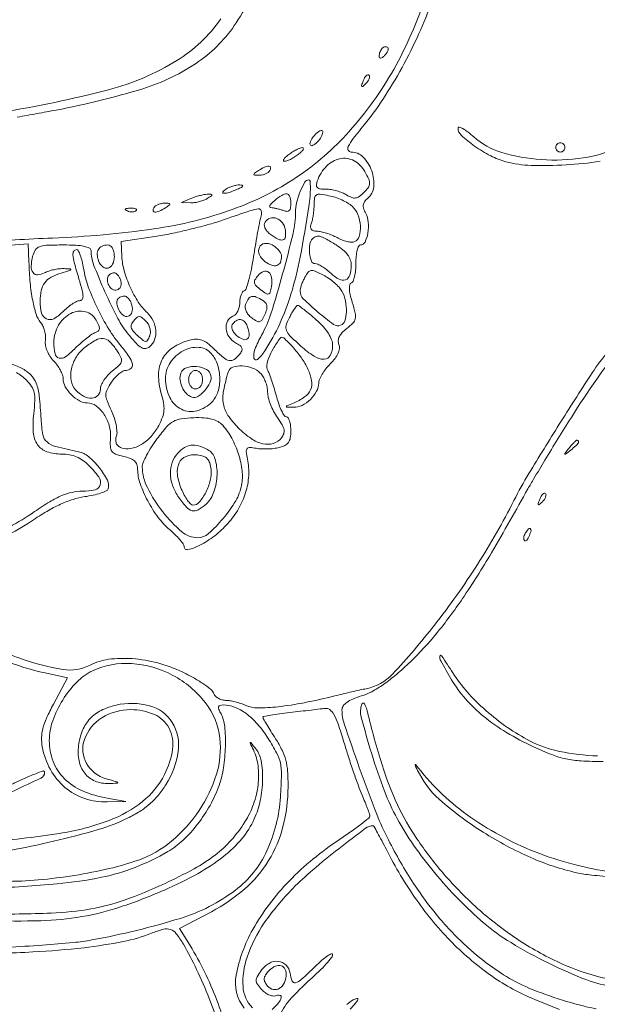
# Model space of a CAD drawing. Units: inches. Extents: x 2656 to 9931, y 1941 to 3068.
# Tile 34 of 46: x 2845.52 to 2854.27, y 2952.23 to 2967.13. Entities that reach past the tile are written whole.
import ezdxf

# ---------------------------------------------------------------- set-up
doc = ezdxf.new("R2010")
doc.units = ezdxf.units.IN
doc.layers.add('A-ANNO-DIMS', color=2, linetype='Continuous', lineweight=18)
doc.layers.add('A-ELEV-ORN', color=8, linetype='Continuous', lineweight=13)
doc.styles.get("Standard").update_dxf_attribs({"font": 'arial.ttf'})
doc.dimstyles.new('ISO-25', dxfattribs={"dimtxt": 6, "dimasz": 2.5, "dimexe": 1.25, "dimexo": 0.625, "dimtad": 1, "dimdec": 0, "dimlunit": 3, "dimtxsty": 'Standard', "dimcen": 2.5, "dimadec": 0, "dimazin": 0, "dimtfac": 1, "dimtdec": 0, "dimtmove": 0, "dimatfit": 3, "dimfxl": 1, "dimarcsym": 0})

# ---------------------------------------------------------------- blocks, each defined once
blk = doc.blocks.new('*D151')
at = {"layer": 'A-ANNO-DIMS', "color": 0, "lineweight": -2, "transparency": 16777216}
for p, q in [((2829.546, 2956.424), (2829.546, 2703.709)), ((2867.059, 2955.98), (2867.059, 2703.709)), ((2832.046, 2704.959), (2864.559, 2704.959))]:
    blk.add_line(p, q, dxfattribs=at)
at = {"layer": 'A-ANNO-DIMS', "color": 0, "transparency": 16777216}
for points in [[(2832.046, 2705.376), (2832.046, 2704.543), (2829.546, 2704.959)], [(2864.559, 2705.376), (2864.559, 2704.543), (2867.059, 2704.959)]]:
    blk.add_solid(points, dxfattribs=at)
at = {"layer": 'Defpoints', "color": 0, "transparency": 16777216}
for p in [(2829.546, 2957.049), (2867.059, 2956.605), (2867.059, 2704.959)]:
    blk.add_point(p, dxfattribs=at)
at = {"layer": 'A-ANNO-DIMS', "color": 0, "transparency": 16777216, "insert": (2848.302, 2708.689), "char_height": 6, "attachment_point": 5}
blk.add_mtext('3\'-1 1/2"', dxfattribs=at)
blk = doc.blocks.new('*D152')
at = {"layer": 'A-ANNO-DIMS', "color": 0, "lineweight": -2, "transparency": 16777216}
for p, q in [((2847.28, 2990.828), (2707.323, 2990.828)), ((2708.573, 2988.328), (2708.573, 2952.971)), ((2847.248, 2950.471), (2707.323, 2950.471))]:
    blk.add_line(p, q, dxfattribs=at)
at = {"layer": 'A-ANNO-DIMS', "color": 0, "transparency": 16777216}
for points in [[(2708.156, 2988.328), (2708.989, 2988.328), (2708.573, 2990.828)], [(2708.156, 2952.971), (2708.989, 2952.971), (2708.573, 2950.471)]]:
    blk.add_solid(points, dxfattribs=at)
at = {"layer": 'Defpoints', "color": 0, "transparency": 16777216}
for p in [(2847.905, 2990.828), (2708.573, 2950.471), (2847.873, 2950.471)]:
    blk.add_point(p, dxfattribs=at)
at = {"layer": 'A-ANNO-DIMS', "color": 0, "transparency": 16777216, "insert": (2704.843, 2970.649), "char_height": 6, "attachment_point": 5, "rotation": 90}
blk.add_mtext('3\'-4 1/2"', dxfattribs=at)
blk = doc.blocks.new('*D153')
at = {"layer": 'A-ANNO-DIMS', "color": 0, "lineweight": -2, "transparency": 16777216}
for p, q in [((2826.64, 2993.722), (2826.64, 2703.709)), ((2829.546, 2956.424), (2829.546, 2703.709)), ((2824.14, 2704.959), (2821.64, 2704.959)), ((2826.64, 2704.959), (2829.546, 2704.959)), ((2832.046, 2704.959), (2851.745, 2704.959))]:
    blk.add_line(p, q, dxfattribs=at)
at = {"layer": 'A-ANNO-DIMS', "color": 0, "transparency": 16777216}
for points in [[(2824.14, 2705.376), (2824.14, 2704.543), (2826.64, 2704.959)], [(2832.046, 2705.376), (2832.046, 2704.543), (2829.546, 2704.959)]]:
    blk.add_solid(points, dxfattribs=at)
at = {"layer": 'Defpoints', "color": 0, "transparency": 16777216}
for p in [(2826.64, 2994.347), (2829.546, 2957.049), (2829.546, 2704.959)]:
    blk.add_point(p, dxfattribs=at)
at = {"layer": 'A-ANNO-DIMS', "color": 0, "transparency": 16777216, "insert": (2843.145, 2708.65), "char_height": 6, "attachment_point": 5}
blk.add_mtext('0\'-3"', dxfattribs=at)
blk = doc.blocks.new('*D154')
at = {"layer": 'A-ANNO-DIMS', "color": 0, "lineweight": -2, "transparency": 16777216}
for p, q in [((2708.573, 2996.847), (2708.573, 2999.347)), ((2826.015, 2994.347), (2707.323, 2994.347)), ((2708.573, 2994.347), (2708.573, 2990.828)), ((2847.28, 2990.828), (2707.323, 2990.828)), ((2708.573, 2988.328), (2708.573, 2954.647))]:
    blk.add_line(p, q, dxfattribs=at)
at = {"layer": 'A-ANNO-DIMS', "color": 0, "transparency": 16777216}
for points in [[(2708.156, 2996.847), (2708.989, 2996.847), (2708.573, 2994.347)], [(2708.156, 2988.328), (2708.989, 2988.328), (2708.573, 2990.828)]]:
    blk.add_solid(points, dxfattribs=at)
at = {"layer": 'Defpoints', "color": 0, "transparency": 16777216}
for p in [(2826.64, 2994.347), (2708.573, 2990.828), (2847.905, 2990.828)]:
    blk.add_point(p, dxfattribs=at)
at = {"layer": 'A-ANNO-DIMS', "color": 0, "transparency": 16777216, "insert": (2704.843, 2970.237), "char_height": 6, "attachment_point": 5, "rotation": 90}
blk.add_mtext('0\'-3 1/2"', dxfattribs=at)

msp = doc.modelspace()

# ---------------------------------------------------------------- linework, layer by layer
at = {"layer": 'A-ELEV-ORN'}
for points in [[(2845.488, 2965.66, 0.001937), (2845.785, 2965.713, 0.002024), (2846.077, 2965.767, 0.02762), (2847.387, 2966.09, 0.077708), (2848.233, 2966.501, 0.09773), (2848.802, 2967.089, 0.062193), (2849.216, 2967.949, 0.059261)], [(2851.685, 2967.523, -0.020457), (2851.452, 2966.917, -0.026412), (2851.187, 2966.383, -0.02755), (2850.877, 2965.898, -0.026024), (2850.511, 2965.441, -0.064031), (2849.714, 2964.749, -0.060807), (2848.755, 2964.267, -0.050453), (2847.555, 2963.968, -0.026486), (2846.021, 2963.83, 0.014791), (2844.896, 2963.755, 0.039833)], [(2845.128, 2963.701), (2845.655, 2963.743), (2845.664, 2963.47, 0.015098), (2845.683, 2963.15, 0.025215), (2845.721, 2962.883, 0.029482), (2845.774, 2962.676, 0.096217), (2845.841, 2962.552, -0.067329), (2845.876, 2962.497, -0.041313), (2845.901, 2962.425, -0.040734), (2845.915, 2962.348, -0.056588), (2845.914, 2962.278, 0.07899), (2845.916, 2962.204, 0.049795), (2845.94, 2962.121, 0.047545), (2845.982, 2962.04, 0.052886), (2846.038, 2961.971, -0.039614), (2846.093, 2961.906, -0.035337), (2846.14, 2961.83, -0.037086), (2846.173, 2961.756, -0.084565), (2846.183, 2961.696, 0.131359), (2846.214, 2961.579, 0.066289), (2846.307, 2961.458, 0.066248), (2846.43, 2961.365, 0.130477), (2846.547, 2961.334, -0.158296), (2846.68, 2961.29, -0.088368), (2846.799, 2961.166, -0.079038), (2846.879, 2960.993, -0.085713), (2846.899, 2960.808, 0.027358), (2846.897, 2960.673, 0.142212), (2846.92, 2960.603, 0.154173), (2846.977, 2960.56, 0.033889), (2847.095, 2960.525, -0.037614), (2847.196, 2960.495, -0.09597), (2847.261, 2960.455, -0.121453), (2847.297, 2960.4, -0.082169), (2847.31, 2960.326, 0.083183), (2847.347, 2960.114, 0.036336), (2847.463, 2959.852, 0.036114), (2847.62, 2959.601, 0.059955), (2847.791, 2959.419, -0.017475), (2847.875, 2959.342, -0.02288), (2847.947, 2959.266, -0.021356), (2847.999, 2959.2, -0.157402), (2848.012, 2959.161, 0.482329), (2848.072, 2959.113, 0.063629), (2848.251, 2959.179, 0.044846), (2848.476, 2959.323, 0.043978), (2848.673, 2959.507, 0.051485), (2848.837, 2959.731, 0.057599), (2848.945, 2959.976, 0.059909), (2848.991, 2960.23, 0.064303), (2848.973, 2960.482, -0.019043), (2848.955, 2960.597, -0.200466), (2848.967, 2960.643, -0.248203), (2849.007, 2960.66, -0.029106), (2849.104, 2960.647, 0.03518), (2849.182, 2960.638, 0.020558), (2849.277, 2960.637, 0.020491), (2849.372, 2960.644, 0.032499), (2849.452, 2960.659, 0.054058), (2849.54, 2960.691, 0.125687), (2849.593, 2960.737, 0.113297), (2849.621, 2960.806, 0.039391), (2849.629, 2960.913, 0.030528), (2849.624, 2960.993, 0.047396), (2849.609, 2961.061, 0.060348), (2849.588, 2961.108, 0.260189), (2849.562, 2961.123, -0.25441), (2849.531, 2961.139, -0.029188), (2849.491, 2961.21, -0.029502), (2849.45, 2961.307, -0.019772), (2849.415, 2961.422, 0.007204), (2849.38, 2961.544, 0.007421), (2849.342, 2961.664, 0.007216), (2849.307, 2961.767, 0.03111), (2849.281, 2961.826, -0.151629), (2849.267, 2961.906, -0.058986), (2849.295, 2962.016, -0.043726), (2849.361, 2962.151, -0.02136), (2849.467, 2962.312, -0.446077), (2849.521, 2962.318, -0.02582), (2849.653, 2962.186, -0.030731), (2849.789, 2962.016, -0.042151), (2849.887, 2961.847, -0.065624), (2849.943, 2961.672, -0.146964), (2849.928, 2961.534, -0.139685), (2849.838, 2961.424, -0.057016), (2849.667, 2961.33, 0.002265), (2849.567, 2961.289, 0.321547), (2849.561, 2961.279, 0.38279), (2849.569, 2961.271, 0.002608), (2849.671, 2961.268, 0.125541), (2849.798, 2961.296, 0.074808), (2849.925, 2961.386, 0.074894), (2850.019, 2961.51, 0.12662), (2850.051, 2961.635, -0.104017), (2850.063, 2961.691, -0.032384), (2850.103, 2961.767, -0.030802), (2850.159, 2961.849, -0.029548), (2850.226, 2961.924, 0.033876), (2850.298, 2962.007, 0.058545), (2850.344, 2962.085, 0.074645), (2850.364, 2962.156, 0.121698), (2850.356, 2962.218, -0.110816), (2850.347, 2962.277, -0.096177), (2850.364, 2962.338, -0.075761), (2850.407, 2962.399, -0.040897), (2850.476, 2962.461, 0.036829), (2850.568, 2962.542, 0.143956), (2850.604, 2962.608, 0.109376), (2850.603, 2962.693, 0.016954), (2850.559, 2962.857, -0.018723), (2850.527, 2962.973, -0.04405), (2850.515, 2963.062, -0.066055), (2850.52, 2963.124, -0.262755), (2850.545, 2963.151, 0.222508), (2850.572, 2963.176, 0.035254), (2850.594, 2963.248, 0.033397), (2850.609, 2963.342, 0.023544), (2850.614, 2963.449, -0.023642), (2850.619, 2963.555, -0.037732), (2850.634, 2963.644, -0.043931), (2850.656, 2963.708, -0.295632), (2850.683, 2963.725, 0.29178), (2850.752, 2963.769, 0.067923), (2850.794, 2963.906, 0.061292), (2850.801, 2964.071, 0.102977), (2850.762, 2964.203, -0.042589), (2850.731, 2964.276, -0.112846), (2850.725, 2964.332, -0.126957), (2850.745, 2964.38, -0.061228), (2850.791, 2964.43, 0.199048), (2850.883, 2964.604, 0.109415), (2850.853, 2964.848, 0.109618), (2850.722, 2965.056, 0.200184), (2850.54, 2965.132, -0.298413), (2850.498, 2965.159, -0.222638), (2850.499, 2965.217, -0.048145), (2850.573, 2965.335, -0.006113), (2850.761, 2965.571, 0.02817), (2851.056, 2965.98, 0.01926), (2851.346, 2966.474, 0.019246), (2851.598, 2966.989, 0.02788), (2851.777, 2967.464, -0.014526)], [(2848.567, 2967.146, -0.103766), (2847.903, 2966.516, -0.074462), (2846.868, 2966.075, -0.024075), (2845.233, 2965.732, 0.023987)], [(2854.6, 2965.209, -0.074881), (2854.055, 2965.042, -0.054125), (2853.419, 2965.017, -0.0559), (2852.822, 2965.125, -0.107645), (2852.399, 2965.36, 0.015979), (2852.308, 2965.435, 0.033182), (2852.231, 2965.486, 0.053925), (2852.178, 2965.509, 0.507729), (2852.161, 2965.497, 0.210529), (2852.211, 2965.383, 0.031431), (2852.411, 2965.222, 0.034984), (2852.655, 2965.075, 0.052971), (2852.885, 2964.985, 0.058384), (2853.265, 2964.929, 0.022857), (2853.796, 2964.937, 0.021823), (2854.311, 2964.991, 0.083985)], [(2854.249, 2952.161, -0.023008), (2853.739, 2952.294, -0.023068), (2853.234, 2952.477, -0.042969), (2852.847, 2952.678, -0.040395), (2852.342, 2953.059, -0.035477), (2851.881, 2953.532, -0.033085), (2851.462, 2954.099, -0.026219), (2851.085, 2954.761, -0.024093), (2850.904, 2955.171, -0.007059), (2850.665, 2955.816, -0.00416), (2850.438, 2956.475, -0.081132), (2850.403, 2956.687, -0.152749), (2850.422, 2956.747, -0.08592), (2850.475, 2956.801, -0.058118), (2850.566, 2956.852, -0.024591), (2850.697, 2956.898, 0.052149), (2850.853, 2956.963, 0.027424), (2851.031, 2957.073, 0.023518), (2851.227, 2957.224, 0.015475), (2851.438, 2957.415, 0.030449), (2851.835, 2957.846, 0.021735), (2852.228, 2958.372, 0.016396), (2852.666, 2959.066, 0.006747), (2853.217, 2960.032, -0.008584), (2853.308, 2960.189, -0.001712), (2853.475, 2960.467, -0.001811), (2853.671, 2960.788, -0.001687), (2853.875, 2961.115, -0.028373), (2854.681, 2962.254, -0.056082)], [(2854.396, 2962.072, 0.025999), (2854.163, 2961.749, 0.003163), (2853.692, 2961.01, 0.003538), (2853.233, 2960.266, 0.019761), (2853.006, 2959.857, -0.025293), (2852.455, 2958.89, -0.024226), (2851.802, 2957.969, -0.021134), (2851.169, 2957.229, -0.158603), (2850.771, 2957.008, 0.005641), (2850.677, 2956.989, 0.002373), (2850.553, 2956.961, 0.002347), (2850.419, 2956.93, 0.003055), (2850.297, 2956.9, -0.012629), (2849.829, 2956.795, -0.021947), (2849.435, 2956.735, -0.024664), (2849.125, 2956.717, -0.10946), (2848.948, 2956.755, 0.02618), (2848.873, 2956.784, 0.019467), (2848.787, 2956.809, 0.019793), (2848.705, 2956.827, 0.041477), (2848.639, 2956.832, -0.074507), (2848.582, 2956.841, -0.064432), (2848.528, 2956.866, -0.066856), (2848.483, 2956.902, -0.09592), (2848.456, 2956.946, 0.135164), (2848.415, 2957.001, 0.019232), (2848.299, 2957.085, 0.020724), (2848.151, 2957.176, 0.016328), (2847.983, 2957.262, 0.045412), (2847.613, 2957.398, 0.046726), (2847.227, 2957.463, 0.050582), (2846.871, 2957.453, 0.0883), (2846.59, 2957.365, -0.163294), (2846.18, 2957.3, -0.042657), (2845.525, 2957.468, -0.038553), (2844.769, 2957.801, -0.030663)], [(2845.302, 2959.316, 0.03899), (2845.705, 2959.546, -0.016354), (2845.935, 2959.692, -0.025518), (2846.142, 2959.8, -0.029603), (2846.332, 2959.874, -0.042475), (2846.508, 2959.915, 0.018492), (2846.637, 2959.938, 0.026143), (2846.749, 2959.969, 0.024598), (2846.835, 2960.002, 0.211487), (2846.862, 2960.032, 0.2024), (2846.852, 2960.165, 0.048072), (2846.729, 2960.354, 0.04877), (2846.565, 2960.522, 0.126447), (2846.414, 2960.596, -0.011877), (2846.069, 2960.674, -0.117882), (2845.938, 2960.743, -0.170367), (2845.875, 2960.853, -0.031647), (2845.848, 2961.089, 0.01358), (2845.82, 2961.439, 0.064726), (2845.773, 2961.633, 0.107185), (2845.691, 2961.759, 0.075435), (2845.553, 2961.859, 0.057839), (2845.366, 2961.93, 0.180103)], [(2845.477, 2961.793, -0.065835), (2845.629, 2961.677, -0.052375), (2845.705, 2961.582, -0.092126), (2845.744, 2961.49, -0.065516), (2845.753, 2961.369, -0.016207), (2845.736, 2961.17, 0.048024), (2845.73, 2960.887, 0.134535), (2845.796, 2960.701, 0.162378), (2845.937, 2960.596, 0.079646), (2846.162, 2960.56, -0.046996), (2846.277, 2960.549, -0.052481), (2846.384, 2960.517, -0.052054), (2846.482, 2960.463, -0.044979), (2846.573, 2960.387, -0.040846), (2846.721, 2960.213, -0.222133), (2846.743, 2960.095, -0.278389), (2846.666, 2960.02, -0.058192), (2846.472, 2959.997, 0.053728), (2846.317, 2959.98, 0.047138), (2846.161, 2959.931, 0.035355), (2845.981, 2959.839, 0.01398), (2845.748, 2959.688, -0.025269), (2845.366, 2959.454, -0.03501)], [(2845.269, 2957.445, 0.045204), (2845.91, 2957.246), (2846.249, 2957.173), (2846.036, 2956.774, 0.015297), (2845.93, 2956.562, 0.043542), (2845.875, 2956.406, 0.058138), (2845.856, 2956.271, 0.050737), (2845.867, 2956.129, 0.08076), (2845.989, 2955.785, 0.091523), (2846.21, 2955.515, 0.093905), (2846.508, 2955.346, 0.090131), (2846.851, 2955.294), (2847.132, 2955.302), (2846.851, 2955.35, -0.060063), (2846.476, 2955.461, -0.094302), (2846.199, 2955.649, -0.105744), (2846.031, 2955.908, -0.092677), (2845.973, 2956.226, -0.084233), (2846.025, 2956.521, -0.053759), (2846.176, 2956.836, -0.054037), (2846.389, 2957.108, -0.089289), (2846.626, 2957.278, -0.12956), (2847.218, 2957.389, -0.104076), (2847.843, 2957.21, -0.105901), (2848.334, 2956.797, -0.138836), (2848.554, 2956.257, -0.101934), (2848.503, 2955.715, -0.073419), (2848.241, 2955.163, -0.071874), (2847.824, 2954.7, -0.089033), (2847.321, 2954.414, -0.027379), (2846.877, 2954.285, -0.017773), (2846.353, 2954.182, -0.017434), (2845.806, 2954.114, -0.021563), (2845.294, 2954.091, 0.019337)], [(2854.272, 2955.99, -0.038832), (2853.696, 2956.059, -0.070977), (2853.251, 2956.215, -0.031899), (2852.908, 2956.422, -0.028892), (2852.581, 2956.678, -0.029711), (2852.297, 2956.961, -0.04108), (2852.08, 2957.248, 0.005134), (2851.912, 2957.507, 0.683993), (2851.885, 2957.501, 0.168909), (2851.898, 2957.43, 0.004262), (2852.063, 2957.142, 0.049361), (2852.273, 2956.854, 0.039427), (2852.549, 2956.589, 0.035646), (2852.893, 2956.346, 0.026402), (2853.304, 2956.127, 0.01732), (2853.578, 2956.01, 0.040071), (2853.793, 2955.946, 0.037153), (2854.024, 2955.915, 0.013073), (2854.359, 2955.904, 0.095042)], [(2845.358, 2954.556, 0.010951), (2846.035, 2954.698, 0.013876), (2846.714, 2954.876, 0.042698), (2847.157, 2955.047, 0.026486), (2847.343, 2955.151, 0.038993), (2847.494, 2955.263, 0.040467), (2847.621, 2955.394, 0.031765), (2847.737, 2955.553, 0.105705), (2847.924, 2956.058, 0.177208), (2847.832, 2956.496, 0.190205), (2847.488, 2956.75, 0.121379), (2846.985, 2956.76, 0.059498), (2846.756, 2956.679, 0.091), (2846.588, 2956.554, 0.092006), (2846.476, 2956.378, 0.062064), (2846.416, 2956.147, 0.082949), (2846.423, 2955.915, 0.11799), (2846.509, 2955.728, 0.12778), (2846.665, 2955.61, 0.107339), (2846.869, 2955.573, 0.002441), (2847.001, 2955.578, 0.534877), (2847.007, 2955.587, 0.215183), (2846.993, 2955.598, 0.001329), (2846.835, 2955.644, -0.194581), (2846.537, 2955.878, -0.218344), (2846.504, 2956.239, -0.170701), (2846.769, 2956.567, -0.139753), (2847.204, 2956.692, -0.1027), (2847.563, 2956.617, -0.172156), (2847.785, 2956.41, -0.157067), (2847.839, 2956.093, -0.082545), (2847.716, 2955.707, -0.106392), (2847.384, 2955.301, -0.078804), (2846.879, 2955.014, -0.051815), (2846.123, 2954.817, -0.017355), (2844.987, 2954.683, 0.004203)], [(2845.058, 2953.984, 0.008566), (2846.094, 2954.055, 0.029332), (2846.762, 2954.153, 0.042246), (2847.274, 2954.304, 0.039474), (2847.765, 2954.542, 0.055678), (2847.998, 2954.716, 0.039563), (2848.218, 2954.958, 0.038179), (2848.406, 2955.242, 0.04122), (2848.543, 2955.545, 0.048745), (2848.61, 2955.812, 0.030311), (2848.638, 2956.135, 0.029611), (2848.628, 2956.437, 0.100228), (2848.572, 2956.626, -0.02464), (2848.539, 2956.695, -0.156991), (2848.536, 2956.734, -0.269337), (2848.556, 2956.755, -0.072224), (2848.604, 2956.762, -0.094583), (2848.777, 2956.729, -0.065244), (2848.953, 2956.631, -0.054803), (2849.125, 2956.472, -0.035883), (2849.286, 2956.256, -0.020267), (2849.414, 2956.037, -0.07093), (2849.47, 2955.884, -0.057405), (2849.486, 2955.706, -0.010213), (2849.472, 2955.37, -0.091557), (2849.266, 2954.553, -0.123706), (2848.791, 2953.96, -0.087858), (2847.957, 2953.532, -0.029294), (2846.618, 2953.205, -0.021888), (2846.337, 2953.166, -0.00529), (2845.869, 2953.127, -0.005418), (2845.331, 2953.093, -0.005359)], [(2848.643, 2951.884, 0.023015), (2848.508, 2952.294, 0.022134), (2848.321, 2952.724, 0.024838), (2848.104, 2953.119), (2847.944, 2953.379), (2848.426, 2953.633, 0.058566), (2848.931, 2953.979, 0.075611), (2849.293, 2954.407, 0.076083), (2849.51, 2954.922, 0.060209), (2849.587, 2955.521, 0.018573), (2849.58, 2955.757, 0.046373), (2849.552, 2955.927, 0.051606), (2849.496, 2956.078, 0.028121), (2849.399, 2956.251, -0.003788), (2849.325, 2956.366, -0.005753), (2849.263, 2956.468, -0.002389), (2849.212, 2956.556, -0.131705), (2849.207, 2956.575, -0.358554), (2849.217, 2956.586, -0.003968), (2849.326, 2956.607, -0.009986), (2849.457, 2956.628, -0.006072), (2849.612, 2956.647, 0.000413), (2849.776, 2956.666, 0.000452), (2849.935, 2956.685, 0.000422), (2850.071, 2956.701, 0.002277), (2850.145, 2956.71, -0.19687), (2850.218, 2956.691, -0.102786), (2850.28, 2956.619, -0.046521), (2850.345, 2956.474, -0.008902), (2850.432, 2956.199, 0.005518), (2850.501, 2955.977, 0.004821), (2850.578, 2955.747, 0.004852), (2850.651, 2955.54, 0.014345), (2850.707, 2955.399, -0.005987), (2850.752, 2955.291, -0.008067), (2850.79, 2955.193, -0.00579), (2850.82, 2955.11, -0.082339), (2850.825, 2955.079, -0.227737), (2850.811, 2955.05, -0.005167), (2850.69, 2954.955, -0.010558), (2850.541, 2954.846, -0.006824), (2850.364, 2954.725, 0.052929), (2849.604, 2954.097, 0.065264), (2849.053, 2953.362, 0.082259), (2848.801, 2952.672, 0.216659), (2848.924, 2952.173, 0.024142)], [(2854.437, 2952.614, -0.051733), (2853.786, 2952.82, -0.039695), (2853.128, 2953.172, -0.037706), (2852.498, 2953.645, -0.035619), (2851.934, 2954.216, -0.028457), (2851.536, 2954.738, -0.038871), (2851.244, 2955.252, -0.034187), (2851.01, 2955.854, -0.016235), (2850.788, 2956.656, 0.022521), (2850.766, 2956.732, 0.068912), (2850.743, 2956.779, 0.245579), (2850.722, 2956.79, 0.315781), (2850.704, 2956.778, 0.153325), (2850.695, 2956.577, 0.010509), (2850.853, 2956.023, 0.01611), (2851.046, 2955.459, 0.034582), (2851.239, 2955.041, 0.027355), (2851.488, 2954.639, 0.020395), (2851.805, 2954.224, 0.019895), (2852.165, 2953.823, 0.021799), (2852.545, 2953.465, 0.042817), (2852.962, 2953.164, 0.021453), (2853.533, 2952.853, 0.020936), (2854.109, 2952.6, 0.063438), (2854.524, 2952.497, 0.048495)], [(2845.048, 2953.501, 0.017732), (2845.842, 2953.496, 0.035466), (2846.466, 2953.558, 0.037714), (2847.05, 2953.705, 0.022995), (2847.714, 2953.96, 0.022415), (2848.224, 2954.212, 0.041687), (2848.608, 2954.467, 0.05125), (2848.887, 2954.738, 0.067354), (2849.076, 2955.039, 0.056201), (2849.167, 2955.317, 0.045577), (2849.202, 2955.63, 0.047702), (2849.181, 2955.914, 0.127027), (2849.098, 2956.098, 0.000877), (2849.022, 2956.193, 0.349364), (2849.014, 2956.194, 0.412352), (2849.011, 2956.187, 0.000946), (2849.063, 2956.081, -0.083658), (2849.133, 2955.839, -0.058663), (2849.133, 2955.554, -0.055445), (2849.064, 2955.261, -0.05641), (2848.933, 2954.991, -0.041061), (2848.725, 2954.715, -0.046828), (2848.482, 2954.49, -0.038405), (2848.163, 2954.282, -0.016986), (2847.714, 2954.056, -0.022131), (2847.107, 2953.807, -0.043487), (2846.603, 2953.675, -0.03345), (2846.003, 2953.612, -0.008488), (2845.025, 2953.593, 0.005699)], [(2854.574, 2954.222, -0.059511), (2853.396, 2954.512, -0.061335), (2852.353, 2955.06, -0.076133), (2851.557, 2955.812, 0.019724), (2851.517, 2955.86, 0.758332), (2851.509, 2955.856, 0.071413), (2851.522, 2955.819, 0.004687), (2851.576, 2955.717, 0.092349), (2851.924, 2955.289, 0.036052), (2852.541, 2954.836, 0.035535), (2853.264, 2954.451, 0.05051), (2853.955, 2954.223, 0.028072), (2854.178, 2954.187, 0.008256), (2854.522, 2954.157, 0.008262)], [(2845.032, 2955.277, 0.002127), (2845.846, 2955.654, 0.291114), (2845.902, 2955.741, 0.521089), (2845.872, 2955.761, 0.011668), (2845.684, 2955.688, 0.013123), (2845.413, 2955.565, 0.004002)], [(2849.048, 2952.178, -0.185893), (2848.905, 2952.5, -0.094612), (2848.967, 2952.945, -0.069796), (2849.227, 2953.462, -0.043177), (2849.661, 2953.986, -0.021681), (2849.958, 2954.262, -0.01078), (2850.356, 2954.586, -0.005042), (2850.76, 2954.895, -0.161985), (2850.876, 2954.933, -0.270899), (2850.886, 2954.927, -0.001508), (2850.941, 2954.827, -0.005801), (2851.004, 2954.711, -0.003584), (2851.075, 2954.573, 0.035539), (2851.534, 2953.808, 0.042363), (2852.074, 2953.162, 0.04546), (2852.676, 2952.655, 0.055612), (2853.322, 2952.304), (2853.698, 2952.151)], [(2843.511, 2952.059, -0.051755), (2843.327, 2952.345, -0.041492), (2843.171, 2952.73, -0.377765), (2843.239, 2952.882, -0.098601), (2843.512, 2952.947, -0.002772), (2844.723, 2952.984, 0.007206), (2845.725, 2953.023, 0.015319), (2846.498, 2953.088, 0.019538), (2847.092, 2953.181, 0.046793), (2847.519, 2953.307, -0.030169), (2847.701, 2953.367, -0.14877), (2847.807, 2953.363, -0.147977), (2847.894, 2953.3, -0.029745), (2848.002, 2953.141, -0.023126), (2848.203, 2952.759, -0.016851), (2848.393, 2952.319, -0.01692), (2848.543, 2951.895, -0.043427)], [(2849.449, 2952.027, -0.093777), (2849.607, 2952.292, -0.031312), (2849.928, 2952.612, 0.012352), (2850.056, 2952.73, 0.017253), (2850.164, 2952.842, 0.013681), (2850.246, 2952.939, 0.170859), (2850.262, 2952.984, 0.540894), (2850.244, 2952.996, 0.046486), (2850.184, 2952.963, 0.029596), (2850.098, 2952.897, 0.014208), (2849.996, 2952.802, -0.007962), (2849.787, 2952.605, -0.120139), (2849.701, 2952.558, -0.376948), (2849.648, 2952.583, -0.062881), (2849.617, 2952.7, 0.155866), (2849.557, 2952.823, 0.180079), (2849.44, 2952.881, 0.153882), (2849.299, 2952.851, 0.112369), (2849.18, 2952.743, 0.023976), (2849.12, 2952.647, 0.135114), (2849.105, 2952.589, 0.148511), (2849.123, 2952.535, 0.030948), (2849.187, 2952.455, 0.049126), (2849.238, 2952.408, 0.054279), (2849.297, 2952.374, 0.061467), (2849.352, 2952.357, 0.136546), (2849.396, 2952.361, -0.144956), (2849.462, 2952.366, -0.422878), (2849.484, 2952.332, -0.117817), (2849.443, 2952.253, -0.031818), (2849.345, 2952.153, -0.02297)], [(2850.525, 2952.156, 0.014705), (2850.609, 2952.248, 0.085937), (2850.643, 2952.304, 0.609614), (2850.629, 2952.32, 0.07342), (2850.574, 2952.297, 0.028686), (2850.476, 2952.229, 0.011691)]]:
    msp.add_lwpolyline(points, format="xyb", dxfattribs=at)
for points in [[(2851.012, 2966.702, 0.063896), (2850.995, 2966.679, 0.039129), (2850.979, 2966.648, 0.038674), (2850.969, 2966.614, 0.054831), (2850.966, 2966.583, 0.142677), (2850.972, 2966.56, 0.290264), (2850.988, 2966.553, 0.131573), (2851.014, 2966.563, 0.034019), (2851.049, 2966.593, 0.041736), (2851.078, 2966.628, 0.061283), (2851.097, 2966.663, 0.080535), (2851.103, 2966.693, 0.212536), (2851.096, 2966.713, 0.128169), (2851.078, 2966.723, 0.100736), (2851.056, 2966.725, 0.089268), (2851.033, 2966.718, 0.075941)], [(2850.724, 2966.207, 0.008399), (2850.7, 2966.14, 0.286372), (2850.703, 2966.124, 0.400052), (2850.717, 2966.124, 0.011214), (2850.763, 2966.168, 0.043285), (2850.794, 2966.204, 0.063152), (2850.813, 2966.241, 0.082976), (2850.82, 2966.272, 0.20742), (2850.811, 2966.294, 0.278911), (2850.792, 2966.299, 0.120343), (2850.769, 2966.285, 0.070189), (2850.745, 2966.253, 0.036269)], [(2849.981, 2965.378, 0.033123), (2849.949, 2965.334, 0.048615), (2849.927, 2965.291, 0.060418), (2849.918, 2965.255, 0.231506), (2849.926, 2965.234, 0.262339), (2849.946, 2965.228, 0.072676), (2849.977, 2965.241, 0.053484), (2850.014, 2965.268, 0.03334), (2850.051, 2965.307, 0.033123), (2850.083, 2965.352, 0.048615), (2850.105, 2965.395, 0.060418), (2850.114, 2965.43, 0.231506), (2850.106, 2965.452, 0.262339), (2850.086, 2965.457, 0.072676), (2850.055, 2965.444, 0.053484), (2850.018, 2965.417, 0.03334)], [(2849.598, 2965.094, 0.02314), (2849.55, 2965.054, 0.065258), (2849.522, 2965.021, 0.206301), (2849.519, 2965.001, 0.344492), (2849.532, 2964.991, 0.091785), (2849.568, 2964.998, 0.024227), (2849.622, 2965.021, 0.023749), (2849.681, 2965.055, 0.022398), (2849.739, 2965.094, 0.02314), (2849.787, 2965.134, 0.065258), (2849.815, 2965.167, 0.206301), (2849.818, 2965.187, 0.344492), (2849.805, 2965.198, 0.091785), (2849.769, 2965.191, 0.024227), (2849.715, 2965.167, 0.023749), (2849.656, 2965.134, 0.022398)], [(2853.638, 2965.202, 0.099038), (2853.644, 2965.175, 0.097945), (2853.659, 2965.152, 0.097945), (2853.682, 2965.137, 0.099038), (2853.709, 2965.132, 0.099038), (2853.735, 2965.137, 0.097945), (2853.758, 2965.152, 0.097945), (2853.774, 2965.175, 0.099038), (2853.779, 2965.202, 0.099038), (2853.774, 2965.229, 0.097945), (2853.758, 2965.252, 0.097945), (2853.735, 2965.267, 0.099038), (2853.709, 2965.272, 0.099038), (2853.682, 2965.267, 0.097945), (2853.659, 2965.252, 0.097945), (2853.644, 2965.229, 0.099038)], [(2850.751, 2964.835, -0.020477), (2850.81, 2964.72, -0.120658), (2850.822, 2964.654, -0.148391), (2850.802, 2964.596, -0.036284), (2850.735, 2964.519, -0.036756), (2850.665, 2964.459, -0.125193), (2850.609, 2964.436, -0.132305), (2850.551, 2964.443, -0.043113), (2850.473, 2964.482, 0.045405), (2850.407, 2964.516, 0.026788), (2850.324, 2964.544, 0.026642), (2850.237, 2964.563, 0.040793), (2850.16, 2964.569, -0.031174), (2850.074, 2964.574, -0.158779), (2850.031, 2964.595, -0.225668), (2850.016, 2964.631, -0.067422), (2850.029, 2964.692, -0.105833), (2850.169, 2964.919, -0.154575), (2850.373, 2965.031, -0.175846), (2850.586, 2964.999, -0.140458)], [(2849.137, 2964.85, 0.010223), (2849.078, 2964.81, 0.295079), (2849.071, 2964.794, 0.343021), (2849.083, 2964.783, 0.012098), (2849.15, 2964.781, 0.053738), (2849.199, 2964.786, 0.049393), (2849.247, 2964.801, 0.052761), (2849.287, 2964.823, 0.101161), (2849.313, 2964.85, 0.175918), (2849.322, 2964.895, 0.372932), (2849.297, 2964.917, 0.110887), (2849.23, 2964.902, 0.03301)], [(2848.645, 2964.569, 0.095694), (2848.601, 2964.527, 0.608383), (2848.612, 2964.507, 0.081911), (2848.693, 2964.52, 0.019739), (2848.82, 2964.569, 0.014925), (2848.88, 2964.597, 0.152377), (2848.899, 2964.615, 0.491407), (2848.893, 2964.628, 0.051935), (2848.856, 2964.633, 0.053798), (2848.808, 2964.63, 0.029384), (2848.75, 2964.616, 0.028934), (2848.693, 2964.595, 0.040566)], [(2849.9, 2964.305, -0.01121), (2849.77, 2963.542, -0.026162), (2849.631, 2962.98, -0.033471), (2849.46, 2962.53, -0.037248), (2849.235, 2962.123, -0.060248), (2849.125, 2961.992, -0.586786), (2849.071, 2962.009, -0.147174), (2849.084, 2962.145, -0.031295), (2849.187, 2962.361, 0.050523), (2849.325, 2962.68, 0.009665), (2849.505, 2963.287, 0.009212), (2849.662, 2963.899, 0.058123), (2849.7, 2964.219, -0.060183), (2849.717, 2964.365, -0.036037), (2849.771, 2964.533, -0.031284), (2849.84, 2964.675, -0.271697), (2849.898, 2964.71, -0.386334), (2849.92, 2964.69, -0.022867), (2849.925, 2964.593, -0.024378), (2849.919, 2964.463, -0.013319)], [(2848.117, 2964.428), (2847.976, 2964.368), (2848.117, 2964.364, 0.04208), (2848.179, 2964.367, 0.028709), (2848.247, 2964.381, 0.029001), (2848.313, 2964.402, 0.050598), (2848.363, 2964.428, 0.006504), (2848.426, 2964.47, 0.247646), (2848.434, 2964.484, 0.411928), (2848.425, 2964.494, 0.011111), (2848.363, 2964.493, 0.038039), (2848.313, 2964.487, 0.016709), (2848.247, 2964.472, 0.016424), (2848.179, 2964.452, 0.021159)], [(2849.629, 2964.35, -0.043546), (2849.623, 2964.283, -0.16083), (2849.604, 2964.246, -0.207384), (2849.569, 2964.234, -0.076984), (2849.518, 2964.245, 0.019483), (2849.469, 2964.261, 0.015062), (2849.415, 2964.276, 0.015308), (2849.364, 2964.286, 0.034964), (2849.325, 2964.29, -0.603928), (2849.31, 2964.32, -0.060327), (2849.38, 2964.395, -0.036603), (2849.491, 2964.476, -0.139342), (2849.572, 2964.499, -0.232987), (2849.594, 2964.488, -0.072284), (2849.613, 2964.455, -0.055156), (2849.625, 2964.407, -0.036553)], [(2850.557, 2964.311, -0.117781), (2850.642, 2964.186, -0.074824), (2850.681, 2964.013, -0.083776), (2850.665, 2963.855, -0.238788), (2850.593, 2963.775, -0.1101), (2850.546, 2963.768, -0.038167), (2850.478, 2963.778, -0.035712), (2850.402, 2963.802, -0.034549), (2850.329, 2963.836, 0.026692), (2850.254, 2963.872, 0.021599), (2850.169, 2963.904, 0.022109), (2850.088, 2963.926, 0.051326), (2850.026, 2963.933, -0.057607), (2849.97, 2963.941, -0.167421), (2849.938, 2963.962, -0.185377), (2849.927, 2963.997, -0.072938), (2849.938, 2964.047, 0.038661), (2849.955, 2964.102, 0.016437), (2849.968, 2964.178, 0.016148), (2849.978, 2964.261, 0.020382), (2849.981, 2964.337, -0.035622), (2849.988, 2964.439, -0.225967), (2850.016, 2964.481, -0.167464), (2850.072, 2964.493, -0.018284), (2850.205, 2964.471, -0.032838), (2850.3, 2964.446, -0.024787), (2850.401, 2964.406, -0.025299), (2850.492, 2964.359, -0.051686)], [(2847.554, 2964.288, 0.175918), (2847.545, 2964.243, 0.372932), (2847.57, 2964.221, 0.110887), (2847.637, 2964.236, 0.03301), (2847.73, 2964.288, 0.010223), (2847.789, 2964.328, 0.295079), (2847.796, 2964.344, 0.343021), (2847.784, 2964.355, 0.012098), (2847.717, 2964.357, 0.053738), (2847.668, 2964.352, 0.049393), (2847.62, 2964.337, 0.052761), (2847.58, 2964.315, 0.101161)], [(2849.179, 2964.165, 0.024458), (2849.161, 2964.09, 0.003403), (2849.13, 2963.933, 0.003888), (2849.097, 2963.747, 0.003289), (2849.065, 2963.549, -0.011655), (2849.031, 2963.359, -0.017445), (2848.992, 2963.195, -0.012536), (2848.952, 2963.063, -0.231808), (2848.922, 2963.033, 0.168506), (2848.897, 2963.013, 0.055194), (2848.875, 2962.969, 0.047691), (2848.86, 2962.911, 0.038325), (2848.856, 2962.847, -0.06012), (2848.848, 2962.782, -0.05988), (2848.825, 2962.721, -0.065554), (2848.79, 2962.672, -0.116301), (2848.75, 2962.645, 0.186203), (2848.671, 2962.573, 0.142758), (2848.649, 2962.457, 0.122649), (2848.693, 2962.333, 0.123637), (2848.79, 2962.246, -0.032782), (2848.861, 2962.201, -0.154993), (2848.889, 2962.163, -0.199615), (2848.887, 2962.122, -0.059536), (2848.851, 2962.067, -0.069487), (2848.769, 2961.992, -0.20567), (2848.695, 2961.977, -0.124398), (2848.608, 2962.02, -0.019891), (2848.468, 2962.149, 0.030321), (2848.368, 2962.238, 0.079176), (2848.284, 2962.284, 0.093687), (2848.199, 2962.298, 0.055144), (2848.096, 2962.284, 0.084339), (2847.847, 2962.174, 0.125219), (2847.687, 2961.999, 0.120802), (2847.626, 2961.763, 0.075208), (2847.667, 2961.479, -0.026347), (2847.702, 2961.333, -0.065796), (2847.708, 2961.223, -0.068943), (2847.686, 2961.119, -0.03122), (2847.629, 2960.99, -0.066467), (2847.514, 2960.826, -0.073984), (2847.364, 2960.704, -0.084926), (2847.204, 2960.643, -0.140969), (2847.062, 2960.656, -0.086125), (2847.015, 2960.684, -0.118974), (2846.987, 2960.723, -0.109346), (2846.978, 2960.773, -0.064777), (2846.989, 2960.834, 0.093997), (2846.997, 2960.902, 0.032388), (2846.984, 2961.001, 0.030838), (2846.955, 2961.111, 0.031159), (2846.913, 2961.216, -0.016217), (2846.846, 2961.369, -0.094862), (2846.829, 2961.455, -0.116244), (2846.847, 2961.533, -0.029742), (2846.912, 2961.646, -0.036972), (2846.965, 2961.715, -0.04027), (2847.026, 2961.773, -0.043964), (2847.086, 2961.813, -0.12723), (2847.134, 2961.826, 0.186281), (2847.208, 2961.855, 0.265161), (2847.23, 2961.92, 0.100189), (2847.182, 2962.033, 0.024359), (2847.058, 2962.195, -0.037279), (2846.873, 2962.452, -0.025178), (2846.7, 2962.769, -0.025439), (2846.563, 2963.092, -0.047404), (2846.492, 2963.367, 0.01957), (2846.47, 2963.478, 0.030173), (2846.442, 2963.57, 0.030312), (2846.411, 2963.639, 0.280016), (2846.385, 2963.655, 0.258861), (2846.343, 2963.631, 0.161629), (2846.329, 2963.575, 0.046641), (2846.35, 2963.459, 0.005632), (2846.422, 2963.209, -0.009193), (2846.471, 2963.036, -0.058325), (2846.483, 2962.946, -0.172925), (2846.468, 2962.9, -0.231085), (2846.43, 2962.881, 0.118254), (2846.384, 2962.87, 0.029573), (2846.317, 2962.831, 0.028548), (2846.244, 2962.775, 0.025323), (2846.174, 2962.71, -0.078005), (2846.04, 2962.609, -0.238281), (2845.93, 2962.606, -0.219075), (2845.855, 2962.695, -0.067956), (2845.832, 2962.872, -0.050838), (2845.85, 2963.037, -0.109237), (2845.903, 2963.153, -0.108996), (2846, 2963.236, -0.050474), (2846.154, 2963.3, 0.002984), (2846.277, 2963.338, 0.179203), (2846.296, 2963.352, 0.567546), (2846.29, 2963.362, 0.00696), (2846.196, 2963.367, 0.038073), (2846.124, 2963.364, 0.025085), (2846.042, 2963.351, 0.025254), (2845.963, 2963.329, 0.043769), (2845.901, 2963.303, -0.106497), (2845.797, 2963.273, -0.258662), (2845.726, 2963.306, -0.169589), (2845.698, 2963.401, -0.049864), (2845.72, 2963.553, -0.077607), (2845.761, 2963.648, -0.166581), (2845.822, 2963.698, -0.079591), (2845.932, 2963.72, -0.009283), (2846.184, 2963.725, -0.012746), (2846.373, 2963.72, -0.03793), (2846.502, 2963.704, -0.061321), (2846.581, 2963.677, -0.288418), (2846.605, 2963.639, 0.092287), (2846.644, 2963.426, 0.013312), (2846.815, 2963.017, 0.015556), (2847.011, 2962.613, 0.051496), (2847.175, 2962.367, 0.01473), (2847.292, 2962.233, 0.074578), (2847.369, 2962.172, 0.158747), (2847.431, 2962.158, 0.148001), (2847.491, 2962.184, 0.135412), (2847.566, 2962.29, 0.103365), (2847.585, 2962.432, 0.095317), (2847.545, 2962.579, 0.095996), (2847.454, 2962.701, -0.066944), (2847.32, 2962.86, -0.036018), (2847.197, 2963.086, -0.035808), (2847.107, 2963.331, -0.058486), (2847.071, 2963.549), (2847.061, 2963.776), (2847.601, 2963.859, 0.013679), (2847.843, 2963.903, 0.008524), (2848.124, 2963.967, 0.008551), (2848.399, 2964.039, 0.015324), (2848.622, 2964.109, -0.002715), (2849.017, 2964.245, -0.056746), (2849.139, 2964.271, -0.369669), (2849.181, 2964.242, -0.137774)], [(2847.154, 2964.24, 0.051402), (2847.193, 2964.229, 0.05415), (2847.232, 2964.226, 0.060344), (2847.266, 2964.232, 0.126455), (2847.289, 2964.245, 0.296942), (2847.292, 2964.261, 0.208169), (2847.28, 2964.274, 0.077125), (2847.246, 2964.281, 0.028489), (2847.197, 2964.282, 0.018894), (2847.144, 2964.278, 0.168741), (2847.124, 2964.268, 0.470617), (2847.125, 2964.255, 0.054073)], [(2849.546, 2963.953, -0.06369), (2849.548, 2963.846, -0.307366), (2849.51, 2963.803, -0.195548), (2849.438, 2963.812, -0.031065), (2849.315, 2963.89, -0.054947), (2849.268, 2963.934, -0.078677), (2849.237, 2963.982, -0.097302), (2849.227, 2964.029, -0.143826), (2849.238, 2964.07, -0.179614), (2849.315, 2964.129, -0.168945), (2849.414, 2964.127, -0.142828), (2849.502, 2964.06, -0.125273)], [(2850.315, 2963.726, -0.034486), (2850.418, 2963.653, -0.063387), (2850.489, 2963.578, -0.076765), (2850.529, 2963.499, -0.081607), (2850.544, 2963.414, -0.071552), (2850.523, 2963.268, -0.234082), (2850.458, 2963.198, -0.219325), (2850.36, 2963.205, -0.064055), (2850.235, 2963.296, 0.024059), (2850.168, 2963.352, 0.026772), (2850.099, 2963.4, 0.027508), (2850.036, 2963.434, 0.110675), (2849.994, 2963.444, -0.314423), (2849.94, 2963.481, -0.063903), (2849.913, 2963.601, -0.059593), (2849.916, 2963.735, -0.162481), (2849.957, 2963.819, -0.11016), (2850.011, 2963.853, -0.151397), (2850.068, 2963.856, -0.065069), (2850.15, 2963.822, -0.008281)], [(2846.957, 2963.549, -0.108196), (2846.931, 2963.434, -0.223085), (2846.863, 2963.376, -0.248588), (2846.781, 2963.395, -0.123502), (2846.718, 2963.485, -0.080341), (2846.698, 2963.58, -0.142552), (2846.716, 2963.657, -0.158361), (2846.771, 2963.707, -0.105871), (2846.855, 2963.725, -0.15208), (2846.896, 2963.712, -0.111514), (2846.929, 2963.677, -0.083213), (2846.95, 2963.621, -0.047734)], [(2849.489, 2963.551, -0.10447), (2849.47, 2963.462, -0.213598), (2849.418, 2963.416, -0.171016), (2849.339, 2963.418, -0.066735), (2849.241, 2963.471, -0.125069), (2849.155, 2963.576, -0.211728), (2849.152, 2963.688, -0.267745), (2849.229, 2963.747, -0.156997), (2849.347, 2963.726, -0.049658), (2849.401, 2963.689, -0.049907), (2849.447, 2963.643, -0.054617), (2849.478, 2963.594, -0.116324)], [(2847.051, 2963.2, -0.144435), (2847.058, 2963.114, -0.207048), (2847.015, 2963.052, -0.232385), (2846.945, 2963.046, -0.164118), (2846.883, 2963.097, -0.089283), (2846.854, 2963.17, -0.132278), (2846.859, 2963.238, -0.162225), (2846.895, 2963.285, -0.150835), (2846.953, 2963.303, -0.143622), (2846.979, 2963.296, -0.059939), (2847.006, 2963.273, -0.052535), (2847.032, 2963.239, -0.046129)], [(2849.336, 2963.096, -0.024594), (2849.318, 2963.01, -0.259111), (2849.294, 2962.984, -0.220238), (2849.257, 2962.989, -0.018187), (2849.175, 2963.045, -0.029349), (2849.102, 2963.106, -0.15873), (2849.078, 2963.15, -0.181623), (2849.086, 2963.196, -0.040811), (2849.133, 2963.263, -0.122481), (2849.217, 2963.325, -0.276204), (2849.292, 2963.313, -0.189719), (2849.338, 2963.231, -0.071773)], [(2850.401, 2963.026, -0.069561), (2850.456, 2962.877, -0.062309), (2850.47, 2962.713, -0.07145), (2850.446, 2962.575, -0.224607), (2850.383, 2962.51, -0.253264), (2850.277, 2962.523, -0.018933), (2850.039, 2962.709, -0.020408), (2849.818, 2962.912, -0.199502), (2849.77, 2963.027, -0.063931), (2849.775, 2963.065, -0.019656), (2849.791, 2963.12, -0.019313), (2849.815, 2963.18, -0.020044), (2849.843, 2963.238, -0.043205), (2849.892, 2963.313, -0.202794), (2849.936, 2963.337, -0.131814), (2849.996, 2963.328, -0.014846), (2850.122, 2963.267, -0.032503), (2850.206, 2963.217, -0.026965), (2850.289, 2963.152, -0.0278), (2850.359, 2963.085, -0.063379)], [(2847.214, 2962.841, -0.117477), (2847.229, 2962.73, -0.225383), (2847.183, 2962.654, -0.280542), (2847.106, 2962.652, -0.142983), (2847.036, 2962.723, -0.058353), (2846.999, 2962.816, -0.145358), (2847.001, 2962.889, -0.197758), (2847.041, 2962.934, -0.118221), (2847.111, 2962.951, -0.14669), (2847.137, 2962.943, -0.059097), (2847.167, 2962.919, -0.051676), (2847.194, 2962.883, -0.044818)], [(2849.203, 2962.885, -0.081328), (2849.246, 2962.847, -0.130802), (2849.266, 2962.802, -0.105067), (2849.263, 2962.746, -0.040709), (2849.237, 2962.673, -0.029647), (2849.195, 2962.592, -0.198787), (2849.16, 2962.565, -0.194038), (2849.115, 2962.571, -0.0281), (2849.037, 2962.622, -0.057001), (2848.985, 2962.67, -0.078764), (2848.951, 2962.725, -0.089584), (2848.938, 2962.781, -0.101923), (2848.947, 2962.836, -0.06571), (2848.989, 2962.912, -0.189763), (2849.039, 2962.944, -0.151832), (2849.106, 2962.937, -0.038327)], [(2850.014, 2962.592, -0.02872), (2850.118, 2962.489, -0.04172), (2850.197, 2962.387, -0.049148), (2850.246, 2962.289, -0.09332), (2850.262, 2962.203, -0.118924), (2850.226, 2962.054, -0.276997), (2850.133, 2961.996, -0.149975), (2849.982, 2962.04, -0.038942), (2849.78, 2962.195, -0.011239), (2849.616, 2962.35, -0.102417), (2849.562, 2962.431, -0.171911), (2849.559, 2962.509, -0.046163), (2849.607, 2962.625, -0.012039), (2849.646, 2962.696, -0.017997), (2849.684, 2962.756, -0.0132), (2849.718, 2962.803, -0.232888), (2849.735, 2962.811, -0.163132), (2849.754, 2962.804, -0.004231), (2849.829, 2962.746, -0.008524), (2849.916, 2962.676, -0.00567)], [(2846.683, 2962.585, -0.02298), (2846.722, 2962.504, -0.119663), (2846.73, 2962.455, -0.206527), (2846.712, 2962.422, -0.089614), (2846.668, 2962.398, 0.070063), (2846.618, 2962.373, 0.015498), (2846.541, 2962.316, 0.015819), (2846.455, 2962.245, 0.014651), (2846.371, 2962.166, -0.034785), (2846.217, 2962.032, -0.229788), (2846.12, 2962.013, -0.287025), (2846.059, 2962.077, -0.048939), (2846.042, 2962.252, -0.132239), (2846.111, 2962.509, -0.142236), (2846.299, 2962.689, -0.183744), (2846.518, 2962.714, -0.211122)], [(2847.492, 2962.349, -0.034637), (2847.461, 2962.282, -0.280553), (2847.432, 2962.265, -0.166296), (2847.394, 2962.28, -0.012056), (2847.307, 2962.355, -0.031101), (2847.241, 2962.422, -0.115621), (2847.214, 2962.475, -0.159927), (2847.217, 2962.524, -0.077358), (2847.25, 2962.579, -0.042512), (2847.298, 2962.627, -0.186187), (2847.335, 2962.641, -0.160823), (2847.375, 2962.626, -0.029853), (2847.435, 2962.573, -0.069924), (2847.472, 2962.524, -0.064019), (2847.496, 2962.465, -0.066362), (2847.503, 2962.404, -0.088171)], [(2848.97, 2962.496, -0.057362), (2849, 2962.38, -0.223762), (2848.978, 2962.31, -0.291098), (2848.918, 2962.294, -0.08162), (2848.826, 2962.34, -0.055198), (2848.779, 2962.384, -0.070949), (2848.747, 2962.433, -0.086794), (2848.734, 2962.48, -0.162098), (2848.743, 2962.519, -0.101043), (2848.8, 2962.579, -0.179915), (2848.865, 2962.596, -0.178969), (2848.925, 2962.566, -0.099927)], [(2846.988, 2962.138, -0.022223), (2847.056, 2962.024, -0.17226), (2847.065, 2961.964, -0.160892), (2847.034, 2961.909, -0.018753), (2846.926, 2961.817, 0.041875), (2846.857, 2961.753, 0.040201), (2846.798, 2961.677, 0.042977), (2846.758, 2961.602, 0.101435), (2846.746, 2961.539, -0.19378), (2846.708, 2961.447, -0.195291), (2846.617, 2961.406, -0.132827), (2846.492, 2961.435, -0.08638), (2846.375, 2961.527, -0.136881), (2846.304, 2961.671, -0.100756), (2846.307, 2961.849, -0.089942), (2846.382, 2962.03, -0.083013), (2846.517, 2962.179, -0.03834), (2846.675, 2962.284, -0.151081), (2846.787, 2962.309, -0.173488), (2846.884, 2962.264, -0.054326)], [(2848.428, 2962.078, -0.096044), (2848.52, 2961.91, -0.074822), (2848.554, 2961.704, -0.077003), (2848.525, 2961.504, -0.11517), (2848.436, 2961.351, -0.138163), (2848.21, 2961.215, -0.183628), (2847.973, 2961.238, -0.166364), (2847.795, 2961.418, -0.113359), (2847.73, 2961.701, -0.146663), (2847.803, 2961.942, -0.123787), (2848, 2962.123, -0.14175), (2848.239, 2962.175, -0.205439)], [(2847.965, 2961.786, 0.119388), (2847.952, 2961.685, 0.080485), (2847.983, 2961.573, 0.081038), (2848.047, 2961.476, 0.124502), (2848.132, 2961.423, 0.222506), (2848.221, 2961.433, 0.072928), (2848.326, 2961.521, 0.070138), (2848.405, 2961.64, 0.159509), (2848.419, 2961.747, 0.224515), (2848.351, 2961.84, 0.103797), (2848.203, 2961.885, 0.103575), (2848.049, 2961.867, 0.223102)], [(2848.293, 2961.685, -0.072314), (2848.285, 2961.631, -0.08892), (2848.262, 2961.586, -0.10214), (2848.228, 2961.555, -0.130775), (2848.187, 2961.545, -0.130775), (2848.147, 2961.555, -0.10214), (2848.113, 2961.586, -0.08892), (2848.09, 2961.631, -0.072314), (2848.082, 2961.685, -0.072314), (2848.09, 2961.739, -0.08892), (2848.113, 2961.785, -0.10214), (2848.147, 2961.815, -0.130775), (2848.187, 2961.826, -0.130775), (2848.228, 2961.815, -0.10214), (2848.262, 2961.785, -0.08892), (2848.285, 2961.739, -0.072314)], [(2849.167, 2961.786, -0.065767), (2849.209, 2961.731, -0.039106), (2849.245, 2961.656, -0.038481), (2849.269, 2961.574, -0.053179), (2849.278, 2961.498, 0.062516), (2849.288, 2961.415, 0.029037), (2849.321, 2961.312, 0.028211), (2849.368, 2961.206, 0.035042), (2849.425, 2961.113, -0.021044), (2849.497, 2961.002, -0.084687), (2849.526, 2960.927, -0.13365), (2849.521, 2960.866, -0.089726), (2849.487, 2960.804, -0.145222), (2849.361, 2960.72, -0.134431), (2849.207, 2960.715, -0.094176), (2849.027, 2960.795, -0.044153), (2848.831, 2960.959, -0.047723), (2848.677, 2961.146, -0.105828), (2848.608, 2961.316, -0.090544), (2848.61, 2961.517, -0.028673), (2848.683, 2961.808, -0.247201), (2848.75, 2961.875, -0.086504), (2848.89, 2961.893, -0.07533), (2849.048, 2961.862, -0.109933)], [(2848.597, 2960.995, -0.061376), (2848.735, 2960.8, -0.046207), (2848.837, 2960.557, -0.047139), (2848.891, 2960.306, -0.075819), (2848.883, 2960.088, -0.088531), (2848.794, 2959.853, -0.039335), (2848.602, 2959.582, -0.037035), (2848.382, 2959.356, -0.183731), (2848.22, 2959.294, -0.180274), (2847.978, 2959.384, -0.048182), (2847.691, 2959.686, -0.048671), (2847.457, 2960.052, -0.114893), (2847.38, 2960.365, -0.105231), (2847.393, 2960.431, -0.020069), (2847.446, 2960.541, -0.020603), (2847.52, 2960.668, -0.017664), (2847.607, 2960.794, -0.018481), (2847.749, 2960.971, -0.084544), (2847.851, 2961.054, -0.095718), (2847.968, 2961.094, -0.027281), (2848.16, 2961.11, -0.023092), (2848.316, 2961.108, -0.048395), (2848.435, 2961.088, -0.06264), (2848.527, 2961.051, -0.082164)], [(2853.84, 2960.648, 0.001576), (2853.778, 2960.568, 0.377591), (2853.779, 2960.56, 0.377591), (2853.787, 2960.559, 0.001576), (2853.867, 2960.621, 0.017685), (2853.941, 2960.684, 0.065617), (2853.981, 2960.731, 0.241985), (2853.983, 2960.757, 0.307699), (2853.963, 2960.771, 0.184603), (2853.949, 2960.765, 0.013803), (2853.916, 2960.735, 0.017649), (2853.879, 2960.695, 0.012436)], [(2847.917, 2960.572, 0.097644), (2847.834, 2960.434, 0.087786), (2847.806, 2960.269, 0.081232), (2847.835, 2960.094, 0.068078), (2847.92, 2959.925, 0.026053), (2848.044, 2959.762, 0.147107), (2848.135, 2959.703, 0.204706), (2848.227, 2959.714, 0.057252), (2848.345, 2959.802, 0.122489), (2848.465, 2959.989, 0.075364), (2848.512, 2960.249, 0.080848), (2848.48, 2960.491, 0.198783), (2848.368, 2960.628, 0.049235), (2848.231, 2960.684, 0.104825), (2848.118, 2960.694, 0.113844), (2848.017, 2960.657, 0.064753)], [(2848.421, 2960.327, -0.091831), (2848.41, 2960.163, -0.054328), (2848.341, 2959.98, -0.055997), (2848.243, 2959.831, -0.223037), (2848.147, 2959.786, -0.207948), (2848.113, 2959.801, -0.033396), (2848.066, 2959.859, -0.03215), (2848.016, 2959.939, -0.02321), (2847.971, 2960.034, -0.064798), (2847.911, 2960.254, -0.144115), (2847.937, 2960.425, -0.190895), (2848.042, 2960.524, -0.124574), (2848.21, 2960.547, -0.049686), (2848.304, 2960.526, -0.123431), (2848.364, 2960.489, -0.119032), (2848.401, 2960.426, -0.04451)], [(2853.397, 2959.877, 0.008399), (2853.372, 2959.81, 0.286372), (2853.376, 2959.794, 0.400052), (2853.39, 2959.794, 0.011214), (2853.436, 2959.838, 0.043285), (2853.467, 2959.874, 0.063152), (2853.486, 2959.911, 0.082976), (2853.493, 2959.942, 0.20742), (2853.484, 2959.964, 0.278911), (2853.465, 2959.969, 0.120343), (2853.442, 2959.955, 0.070189), (2853.418, 2959.923, 0.036269)], [(2853.178, 2959.36, 0.049364), (2853.163, 2959.328, 0.059701), (2853.155, 2959.297, 0.070517), (2853.156, 2959.269, 0.156651), (2853.165, 2959.251, 0.281567), (2853.182, 2959.247, 0.118528), (2853.201, 2959.259, 0.069269), (2853.222, 2959.287, 0.035865), (2853.241, 2959.326, 0.029555), (2853.265, 2959.404, 0.344086), (2853.253, 2959.431, 0.36195), (2853.225, 2959.426, 0.030391)], [(2849.559, 2952.691, -0.100088), (2849.533, 2952.562, -0.148102), (2849.459, 2952.473, -0.195844), (2849.365, 2952.455, -0.17375), (2849.278, 2952.506, -0.044794), (2849.238, 2952.564, -0.128264), (2849.225, 2952.612, -0.129111), (2849.238, 2952.659, -0.045662), (2849.278, 2952.718, -0.083416), (2849.37, 2952.797, -0.161197), (2849.464, 2952.819, -0.223398), (2849.532, 2952.779, -0.150503)]]:
    msp.add_lwpolyline(points, format="xyb", close=True, dxfattribs=at)

# ---------------------------------------------------------------- dimensions: what is measured, and where the dimension line sits
at = {"layer": 'A-ANNO-DIMS'}
for base, p1, p2, picture, middle in [((2708.573, 2990.828), (2826.64, 2994.347), (2847.905, 2990.828), '*D154', (2704.843, 2970.237)), ((2708.573, 2950.471), (2847.905, 2990.828), (2847.873, 2950.471), '*D152', (2704.843, 2970.649))]:
    dim = msp.add_linear_dim(base=base, p1=p1, p2=p2, angle=90, dimstyle='ISO-25', override={"dimdec": 1, "dimlfac": 1, "dimrnd": 0, "dimzin": 1, "dimdsep": 46, "dimlunit": 4, "dimfrac": 2}, dxfattribs=at)
    dim.commit()
    dim.dimension.update_dxf_attribs({"geometry": picture, "text_midpoint": middle})
for base, p1, p2, picture, middle in [((2829.546, 2704.959), (2826.64, 2994.347), (2829.546, 2957.049), '*D153', (2843.145, 2708.65)), ((2867.059, 2704.959), (2829.546, 2957.049), (2867.059, 2956.605), '*D151', (2848.302, 2708.689))]:
    dim = msp.add_linear_dim(base=base, p1=p1, p2=p2, dimstyle='ISO-25', override={"dimdec": 1, "dimlfac": 1, "dimrnd": 0, "dimzin": 1, "dimdsep": 46, "dimlunit": 4, "dimfrac": 2}, dxfattribs=at)
    dim.commit()
    dim.dimension.update_dxf_attribs({"geometry": picture, "text_midpoint": middle})

doc.saveas('drawing.dxf')
